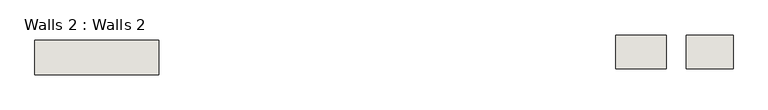
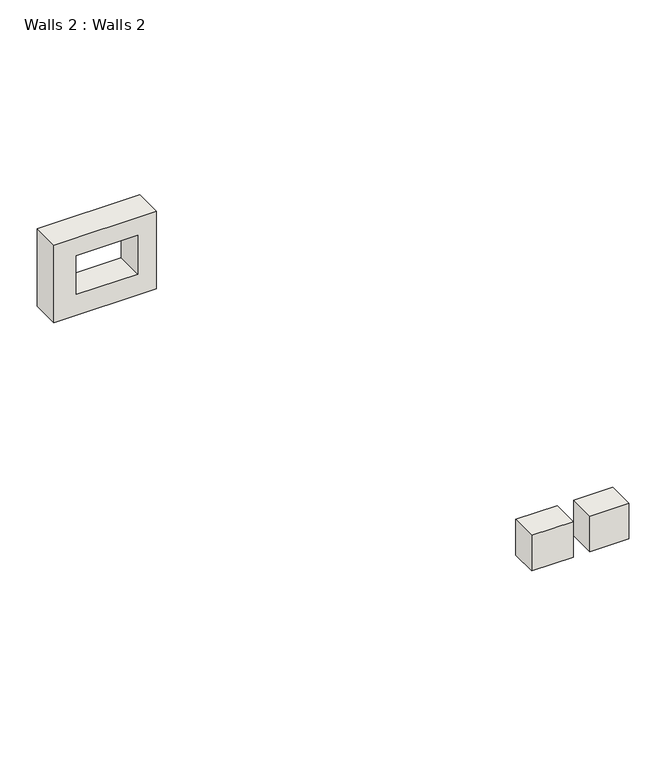
"""IFC4 building model written with IfcOpenShell, lengths in millimetres: wall geometry, Walls 2 : Walls 2."""

from ifc_helpers import new_model, si_unit, frame, origin, place, context, project, spatial, polyline, outline, extrude, source, transform, mapped, element, save


def walls_2_walls_2_2f288bc8(model_context):
    return source(origin(), model_context, "Body", "SweptSolid", [
        extrude(outline(polyline([(-5816.2738398, 1459.0172162), (-6128.1170469, 1459.0172162), (-6128.1170469, 1665.9143948), (-5816.2738398, 1665.9143948), (-5816.2738398, 1459.0172162)])), frame((0.0, 0.0, 5061.9541744), z_axis=(0.0, 0.0, 1.0), x_axis=(1.0, 0.0, 0.0)), (0.0, 0.0, 1.0), 280.3164849),
        extrude(outline(polyline([(-5405.2096624, 1459.0172162), (-5694.9093643, 1459.0172162), (-5694.9093643, 1665.9143948), (-5405.2096624, 1665.9143948), (-5405.2096624, 1459.0172162)])), frame((0.0, 0.0, 5061.9541744), z_axis=(0.0, 0.0, 1.0), x_axis=(1.0, 0.0, 0.0)), (0.0, 0.0, 1.0), 280.3164849),
        extrude(outline(polyline([(8904.3757388, -8946.1093643), (8904.3757388, -9708.1093643), (8294.7757388, -9708.1093643), (8294.7757388, -8946.1093643), (8904.3757388, -8946.1093643)]), holes=[polyline([(8762.2045537, -9084.7800429), (8457.4045537, -9084.7800429), (8457.4045537, -9541.9800429), (8762.2045537, -9541.9800429), (8762.2045537, -9084.7800429)])]), frame((0.0, 1420.7887046, 0.0), z_axis=(0.0, 1.0, 0.0), x_axis=(0.0, 0.0, 1.0)), (0.0, 0.0, 1.0), 212.194009),
    ])


if __name__ == "__main__":
    model = new_model("IFC4")
    model_context = context("Model", 3, world=origin())
    ifc_project = project(units=[si_unit("LENGTHUNIT", "METRE", prefix="MILLI")], contexts=[model_context])
    site = spatial("IfcSite", under=ifc_project)
    building = spatial("IfcBuilding", under=site)
    placement = place(None, origin())
    walls_2_walls_2_shape = walls_2_walls_2_2f288bc8(model_context)
    element("IfcWall", 1, ObjectType="Walls 2 : Walls 2", at=placement, inside=building, context=model_context, shape_type="MappedRepresentation", body=[
        mapped(walls_2_walls_2_shape, transform((0.0, 0.0, 0.0), x_axis=(1.0, 0.0, 0.0), y_axis=(0.0, 1.0, 0.0), z_axis=(0.0, 0.0, 1.0))),
    ])
    save(model, "model.ifc")

# Revit data of these elements
# Element 1 (IfcWall, "Walls 2 : Walls 2")
#   Materials on its faces: "Default Wall"
# Materials
#   "Default Wall": colour RGB 128 128 128, transparency 0
